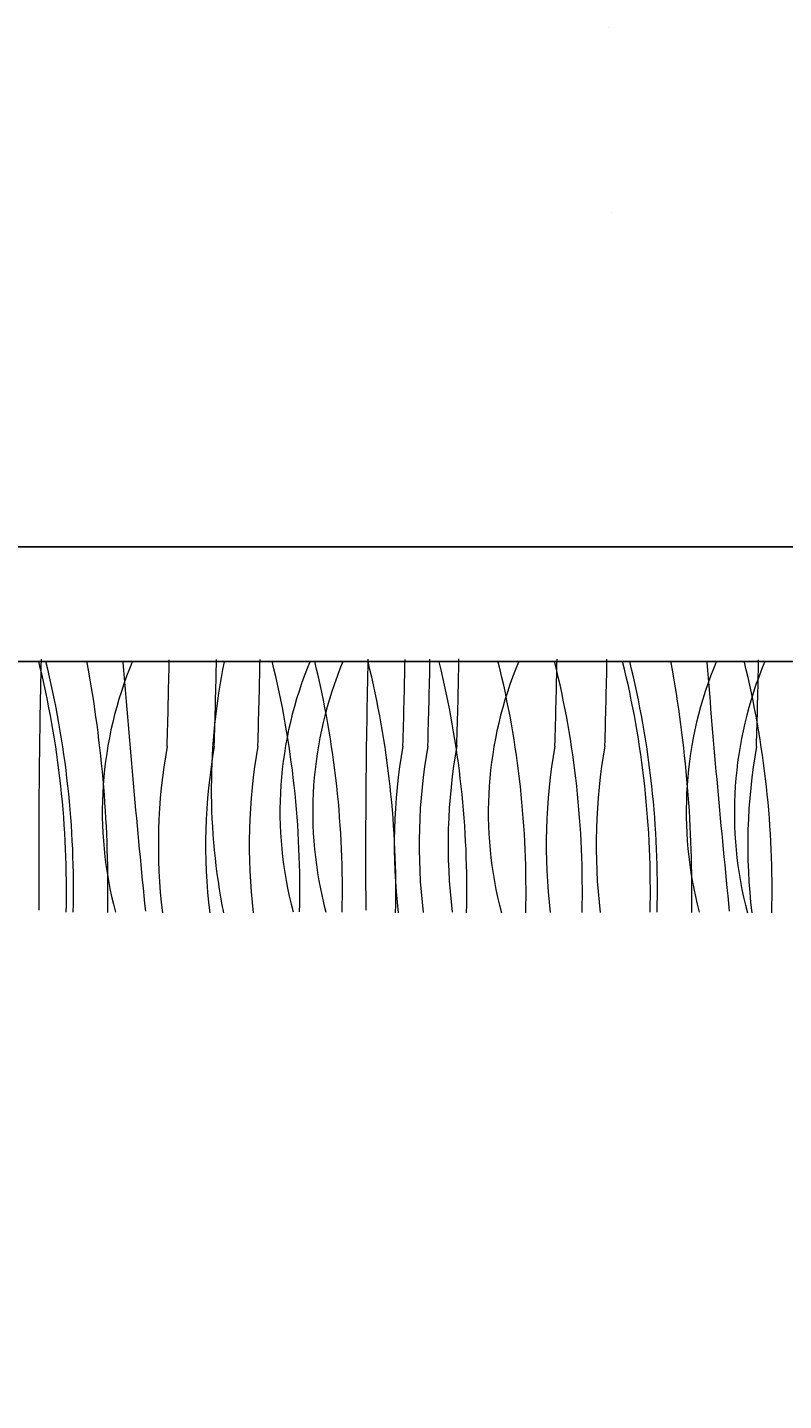
# Model space of a CAD drawing. Units: inches. Extents: x 182 to 1022, y -617 to 111.
# Tile 10 of 33: x 363 to 381, y -308 to -277. Entities that reach past the tile are written whole.
import ezdxf

# ---------------------------------------------------------------- set-up
doc = ezdxf.new("R2010")
doc.units = ezdxf.units.IN
doc.header["$MEASUREMENT"] = 0
doc.layers.add('A-ANNO-DIMS', color=2, linetype='Continuous', lineweight=18)
doc.layers.add('furniture', color=50, linetype='Continuous', lineweight=15, transparency=0.8)
doc.styles.get("Standard").update_dxf_attribs({"font": 'arial.ttf'})
doc.dimstyles.get("Standard").update_dxf_attribs({"dimtxt": 0.18, "dimasz": 0.18, "dimexe": 0.18, "dimexo": 0.0625, "dimgap": 0.09, "dimtad": 0, "dimtih": 1, "dimtoh": 1, "dimdec": 1, "dimzin": 0, "dimdsep": 46, "dimlunit": 4, "dimtxsty": 'Standard', "dimcen": 0.09, "dimadec": 0, "dimazin": 0, "dimtfac": 1, "dimtdec": 1, "dimtofl": 0, "dimtmove": 0, "dimatfit": 3, "dimfxl": 1, "dimtolj": 1, "dimtzin": 0, "dimarcsym": 0})

# ---------------------------------------------------------------- blocks, each defined once
blk = doc.blocks.new('LOUNGE-SEATING-GROUP')
for p, q in [((118.707, 20.037), (118.707, 20.037)), ((118.77, 15.843), (118.77, 15.843)), ((134.145, 5.694), (21.664, 5.694)), ((39.442, 5.694), (134.145, 5.694))]:
    blk.add_line(p, q)
for centre, radius, start, end in [((290.339, 1.329), 184.521, 178.62796, 180.39341), ((84.891, 0.531), 21.554, 358.6331, 13.8573), ((85.051, 0.532), 21.554, 358.6331, 13.8573), ((78.765, 0.5), 28.62, 359.0195, 10.4039), ((116.093, 2.289), 8.837, 157.3098, 194.8613), ((358.539, 25.472), 251.596, 184.51462, 185.80171), ((-33.921, 8.279), 142.714, 358.18909, 358.97752), ((124.055, 2.803), 14.333, 168.4112, 191.2455), ((-32.852, 8.282), 142.714, 358.18909, 358.97752), ((-31.866, 8.285), 142.714, 358.18909, 358.97752), ((90.173, 0.538), 21.554, 358.6331, 13.8573), ((120.114, 2.293), 8.837, 157.3098, 194.8613), ((120.856, 2.285), 8.837, 157.3098, 194.8613), ((91.136, 0.53), 21.554, 358.6331, 13.8573), ((297.736, 1.329), 184.521, 178.62796, 180.39341), ((92.345, 0.521), 21.554, 358.6331, 13.8573), ((-28.584, 8.286), 142.714, 358.18909, 358.97752), ((-28.019, 8.287), 142.714, 358.18909, 358.97752), ((93.953, 0.518), 21.554, 358.6331, 13.8573), ((-27.364, 8.298), 142.714, 358.18909, 358.97752), ((124.829, 2.27), 8.837, 157.3098, 194.8613), ((95.292, 0.516), 21.554, 358.6331, 13.8573), ((96.567, 0.526), 21.554, 358.6331, 13.8573), ((-25.144, 8.289), 142.714, 358.18909, 358.97752), ((-24.013, 8.292), 142.714, 358.18909, 358.97752), ((98.106, 0.531), 21.554, 358.6331, 13.8573), ((98.266, 0.532), 21.554, 358.6331, 13.8573), ((91.98, 0.5), 28.62, 359.0195, 10.4039), ((129.308, 2.289), 8.837, 157.3098, 194.8613), ((371.754, 25.472), 251.596, 184.51462, 185.80171), ((130.398, 2.27), 8.837, 157.3098, 194.8613), ((100.861, 0.516), 21.554, 358.6331, 13.8573), ((-20.582, 8.279), 142.714, 358.18909, 358.97752), ((121.319, 1.534), 12.794, 169.9349, 186.8829), ((122.388, 1.536), 12.794, 169.9349, 186.8829), ((123.374, 1.539), 12.794, 169.9349, 186.8829), ((126.656, 1.54), 12.794, 169.9349, 186.8829), ((127.221, 1.542), 12.794, 169.9349, 186.8829), ((127.876, 1.552), 12.794, 169.9349, 186.8829), ((130.096, 1.543), 12.794, 169.9349, 186.8829), ((131.227, 1.546), 12.794, 169.9349, 186.8829), ((134.658, 1.534), 12.794, 169.9349, 186.8829)]:
    blk.add_arc(centre, radius, start, end)
blk = doc.blocks.new('*D26')
at = {"layer": 'A-ANNO-DIMS', "color": 0, "lineweight": -2, "transparency": 16777216}
for p, q in [((257.848, -296.884), (257.848, -319.733)), ((409.388, -296.884), (409.388, -319.733)), ((258.028, -319.553), (331.642, -319.553)), ((409.208, -319.553), (335.594, -319.553))]:
    blk.add_line(p, q, dxfattribs=at)
at = {"layer": 'A-ANNO-DIMS', "color": 0, "transparency": 16777216}
for points in [[(258.028, -319.523), (258.028, -319.583), (257.848, -319.553)], [(409.208, -319.523), (409.208, -319.583), (409.388, -319.553)]]:
    blk.add_solid(points, dxfattribs=at)
at = {"layer": 'Defpoints', "color": 0, "transparency": 16777216}
for p in [(257.848, -296.822), (409.388, -296.822), (409.388, -319.553)]:
    blk.add_point(p, dxfattribs=at)
at = {"layer": 'A-ANNO-DIMS', "color": 0, "transparency": 16777216, "insert": (333.618, -319.553), "char_height": 0.18, "attachment_point": 5}
blk.add_mtext('\\A1;LOUNGE GROUP 12\'-7 1/2" TYP.', dxfattribs=at)
blk = doc.blocks.new('*D39')
at = {"layer": 'A-ANNO-DIMS', "color": 0, "lineweight": -2, "transparency": 16777216}
for p, q in [((238.398, -288.54), (1015.285, -288.54)), ((1015.105, -288.72), (1015.105, -346.775)), ((1015.105, -405.193), (1015.105, -347.138)), ((238.427, -405.373), (1015.285, -405.373))]:
    blk.add_line(p, q, dxfattribs=at)
at = {"layer": 'A-ANNO-DIMS', "color": 0, "transparency": 16777216}
for points in [[(1015.075, -288.72), (1015.135, -288.72), (1015.105, -288.54)], [(1015.075, -405.193), (1015.135, -405.193), (1015.105, -405.373)]]:
    blk.add_solid(points, dxfattribs=at)
at = {"layer": 'Defpoints', "color": 0, "transparency": 16777216}
for p in [(238.335, -288.54), (1015.105, -288.54), (238.364, -405.373)]:
    blk.add_point(p, dxfattribs=at)
at = {"layer": 'A-ANNO-DIMS', "color": 0, "transparency": 16777216, "insert": (1015.105, -346.956), "char_height": 0.18, "attachment_point": 5}
blk.add_mtext('\\A1;9\'-9"', dxfattribs=at)

msp = doc.modelspace()

# ---------------------------------------------------------------- block references
at = {"layer": 'furniture'}
msp.add_blockref('LOUNGE-SEATING-GROUP', (257.848, -296.822), dxfattribs=at)

# ---------------------------------------------------------------- dimensions: what is measured, and where the dimension line sits
at = {"layer": 'A-ANNO-DIMS'}
dim = msp.add_linear_dim(base=(1015.105, -288.54), p1=(238.364, -405.373), p2=(238.335, -288.54), angle=90, dimstyle='Standard', override={"dimdec": 1, "dimlfac": 1, "dimrnd": 0, "dimzin": 1, "dimdsep": 46, "dimlunit": 4, "dimfrac": 2}, dxfattribs=at)
dim.commit()
dim.dimension.update_dxf_attribs({"geometry": '*D39', "text_midpoint": (1015.105, -346.956)})
dim = msp.add_linear_dim(base=(409.388, -319.553), p1=(257.848, -296.822), p2=(409.388, -296.822), text='LOUNGE GROUP <> TYP.', dimstyle='Standard', override={"dimdec": 1, "dimlfac": 1, "dimrnd": 0, "dimzin": 1, "dimdsep": 46, "dimlunit": 4, "dimfrac": 2}, dxfattribs=at)
dim.commit()
dim.dimension.update_dxf_attribs({"geometry": '*D26', "text_midpoint": (333.618, -319.553)})

doc.saveas('drawing.dxf')
